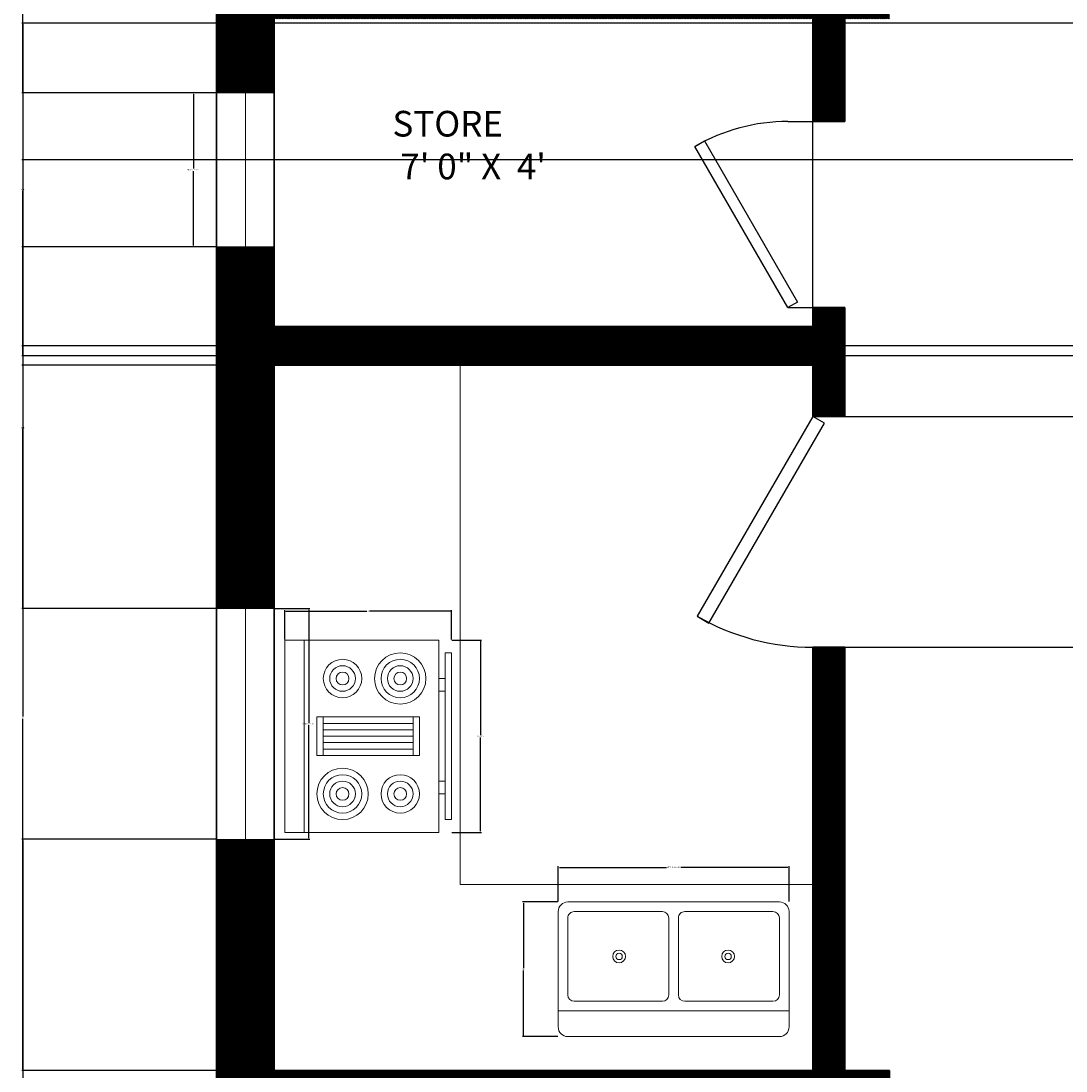
# Model space of a CAD drawing. Units: inches. Extents: x -24 to 516, y -23 to 640.
# Tile 2 of 5: x -24 to 139, y 288 to 452. Entities that reach past the tile are written whole.
import ezdxf

# ---------------------------------------------------------------- set-up
doc = ezdxf.new("R2010")
doc.units = ezdxf.units.IN
doc.header["$MEASUREMENT"] = 0
for name, color, linetype, lineweight in [('A-ANNO-DIMS', 2, 'Continuous', 18), ('A-AREA-IDEN', 7, 'Continuous', 18), ('A-WALL', 7, 'Continuous', 35), ('doors', 40, 'Continuous', 25), ('kitchen', 181, 'Continuous', 18), ('window', 30, 'Continuous', 18)]:
    doc.layers.add(name, color=color, linetype=linetype, lineweight=lineweight)
doc.layers.add('A-WALL-PATT', color=198, linetype='Continuous', lineweight=13, true_color=0x2e0f2e)
doc.styles.get("Standard").update_dxf_attribs({"font": 'arial.ttf'})
doc.dimstyles.get("Standard").update_dxf_attribs({"dimtxt": 0.18, "dimasz": 0.18, "dimexe": 0.18, "dimexo": 0.0625, "dimgap": 0.09, "dimtad": 0, "dimtih": 1, "dimtoh": 1, "dimdec": 4, "dimzin": 0, "dimdsep": 46, "dimtxsty": 'Standard', "dimcen": 0.09, "dimadec": 0, "dimazin": 0, "dimtfac": 1, "dimtdec": 4, "dimtofl": 0, "dimtmove": 0, "dimatfit": 3, "dimfxl": 1, "dimtolj": 1, "dimtzin": 0, "dimarcsym": 0})

# ---------------------------------------------------------------- blocks, each defined once
blk = doc.blocks.new('*U6')
for p, q in [((0, 0), (0, -100)), ((750, 0), (750, -100))]:
    blk.add_line(p, q)
blk.add_lwpolyline([(0, 0), (649.5, 375), (671.4, 337.1), (21.9, -37.9)], close=True)
blk.add_arc((0, 0), 750, 0, 30)
blk = doc.blocks.new('*U7')
for p, q in [((0, 0), (0, 100)), ((750, 0), (750, 100))]:
    blk.add_line(p, q)
blk.add_lwpolyline([(0, 0), (649.5, -375), (671.4, -337.1), (21.9, 37.9)], close=True)
blk.add_arc((0, 0), 750, 330, 0)
blk = doc.blocks.new('Range-Oven - 30 in top')
for p, q in [((0, -3), (30, -3)), ((12, -6), (18, -6)), ((13, -20), (13, -6)), ((14, -6), (14, -20)), ((15, -20), (15, -6)), ((16, -6), (16, -20)), ((17, -20), (17, -6)), ((18, -20), (12, -20)), ((6, -24), (6, -25)), ((8, -25), (8, -24)), ((22, -25), (22, -24)), ((24, -24), (24, -25))]:
    blk.add_line(p, q)
for points in [[(0, -24), (0, 0), (30, 0), (30, -24)], [(12, -21), (12, -5), (18, -5), (18, -21)], [(2, -26), (2, -25), (28, -25), (28, -26)]]:
    blk.add_lwpolyline(points, close=True)
for centre, radius in [((6, -9), 4), ((6, -9), 3), ((24, -9), 3), ((6, -9), 2), ((6, -9), 1), ((24, -9), 2), ((24, -9), 1), ((24, -18), 4), ((6, -18), 3), ((6, -18), 2), ((24, -18), 3), ((24, -18), 2), ((6, -18), 1), ((24, -18), 1)]:
    blk.add_circle(centre, radius)
blk = doc.blocks.new('Sink-double - 36 in top')
for p, q in [((-18, -4), (18, -4)), ((-0.75, -18.5), (-0.75, -6.5)), ((0.75, -6.5), (0.75, -18.5))]:
    blk.add_line(p, q)
for points in [[(-16.5, 0), (16.5, 0)], [(-18, -19.5), (-18, -1.5)], [(18, -1.5), (18, -19.5)], [(-16.5, -18.5), (-16.5, -6.5)], [(-15.5, -5.5), (-1.75, -5.5)], [(1.75, -5.5), (15.5, -5.5)], [(16.5, -6.5), (16.5, -18.5)], [(-1.75, -19.5), (-15.5, -19.5)], [(15.5, -19.5), (1.75, -19.5)], [(16.5, -21), (-16.5, -21)]]:
    blk.add_lwpolyline(points)
for centre, radius in [((-8.5, -12.5), 1), ((-8.5, -12.5), 0.5), ((8.5, -12.5), 1), ((8.5, -12.5), 0.5)]:
    blk.add_circle(centre, radius)
for centre, radius, start, end in [((-16.5, -1.5), 1.5, 90, 180), ((16.5, -1.5), 1.5, 0, 90), ((-15.5, -6.5), 1, 90, 180), ((-1.75, -6.5), 1, 0, 90), ((1.75, -6.5), 1, 90, 180), ((15.5, -6.5), 1, 0, 90), ((-16.5, -19.5), 1.5, 180, 270), ((-15.5, -18.5), 1, 180, 270), ((-1.75, -18.5), 1, 270, 0), ((1.75, -18.5), 1, 180, 270), ((15.5, -18.5), 1, 270, 0), ((16.5, -19.5), 1.5, 270, 0)]:
    blk.add_arc(centre, radius, start, end)
blk = doc.blocks.new('WIN-36IN')
for p, q in [((0, 0), (0, 36)), ((0, 36), (9, 36)), ((4.5, 0), (4.5, 36)), ((9, 36), (9, 0)), ((9, 0), (0, 0)), ((9, 0), (4.5, 0))]:
    blk.add_line(p, q)
blk = doc.blocks.new('WIN-24IN')
for p, q in [((0, 0), (0, 24)), ((0, 24), (9, 24)), ((4.5, 0), (4.5, 24)), ((9, 24), (9, 0)), ((9, 0), (0, 0)), ((9, 0), (4.5, 0))]:
    blk.add_line(p, q)
blk = doc.blocks.new('*D19')
at = {"layer": 'A-ANNO-DIMS', "color": 0, "lineweight": -2, "transparency": 16777216}
for p, q in [((15.15, 360.05), (20.67, 360.05)), ((20.49, 359.87), (20.49, 342.23)), ((20.49, 324.23), (20.49, 341.86)), ((15.15, 324.05), (20.67, 324.05))]:
    blk.add_line(p, q, dxfattribs=at)
at = {"layer": 'A-ANNO-DIMS', "color": 0, "transparency": 16777216}
for points in [[(20.46, 359.87), (20.52, 359.87), (20.49, 360.05)], [(20.46, 324.23), (20.52, 324.23), (20.49, 324.05)]]:
    blk.add_solid(points, dxfattribs=at)
at = {"layer": 'Defpoints', "color": 0, "transparency": 16777216}
for p in [(15.09, 360.05), (20.49, 360.05), (15.09, 324.05)]:
    blk.add_point(p, dxfattribs=at)
at = {"layer": 'A-ANNO-DIMS', "color": 0, "transparency": 16777216, "insert": (20.49, 342.05), "char_height": 0.18, "attachment_point": 5}
blk.add_mtext('\\A1;WINDOW 36 TYP.', dxfattribs=at)
blk = doc.blocks.new('*D20')
at = {"layer": 'A-ANNO-DIMS', "color": 0, "lineweight": -2, "transparency": 16777216}
for p, q in [((6.09, 323.98), (6.09, 318.47)), ((15.09, 323.98), (15.09, 318.47)), ((6.27, 318.65), (10.13, 318.65)), ((14.91, 318.65), (11.05, 318.65))]:
    blk.add_line(p, q, dxfattribs=at)
at = {"layer": 'A-ANNO-DIMS', "color": 0, "transparency": 16777216}
for points in [[(6.27, 318.68), (6.27, 318.62), (6.09, 318.65)], [(14.91, 318.68), (14.91, 318.62), (15.09, 318.65)]]:
    blk.add_solid(points, dxfattribs=at)
at = {"layer": 'Defpoints', "color": 0, "transparency": 16777216}
for p in [(6.09, 324.05), (15.09, 324.05), (15.09, 318.65)]:
    blk.add_point(p, dxfattribs=at)
at = {"layer": 'A-ANNO-DIMS', "color": 0, "transparency": 16777216, "insert": (10.59, 318.65), "char_height": 0.18, "attachment_point": 5}
blk.add_mtext('\\A1;9 TYP.', dxfattribs=at)
blk = doc.blocks.new('*D21')
at = {"layer": 'A-ANNO-DIMS', "color": 0, "lineweight": -2, "transparency": 16777216}
for p, q in [((6.03, 440.47), (2.31, 440.47)), ((2.49, 440.29), (2.49, 428.66)), ((2.49, 416.65), (2.49, 428.29)), ((6.03, 416.47), (2.31, 416.47))]:
    blk.add_line(p, q, dxfattribs=at)
at = {"layer": 'A-ANNO-DIMS', "color": 0, "transparency": 16777216}
for points in [[(2.46, 440.29), (2.52, 440.29), (2.49, 440.47)], [(2.46, 416.65), (2.52, 416.65), (2.49, 416.47)]]:
    blk.add_solid(points, dxfattribs=at)
at = {"layer": 'Defpoints', "color": 0, "transparency": 16777216}
for p in [(2.49, 440.47), (6.09, 440.47), (6.09, 416.47)]:
    blk.add_point(p, dxfattribs=at)
at = {"layer": 'A-ANNO-DIMS', "color": 0, "transparency": 16777216, "insert": (2.49, 428.47), "char_height": 0.18, "attachment_point": 5}
blk.add_mtext('\\A1;WINDOW 24 TYP.', dxfattribs=at)
blk = doc.blocks.new('*D22')
at = {"layer": 'A-ANNO-DIMS', "color": 0, "lineweight": -2, "transparency": 16777216}
for p, q in [((6.09, 440.54), (6.09, 444.25)), ((6.27, 444.07), (10.13, 444.07)), ((14.91, 444.07), (11.05, 444.07)), ((15.09, 440.54), (15.09, 444.25))]:
    blk.add_line(p, q, dxfattribs=at)
at = {"layer": 'A-ANNO-DIMS', "color": 0, "transparency": 16777216}
for points in [[(6.27, 444.1), (6.27, 444.04), (6.09, 444.07)], [(14.91, 444.1), (14.91, 444.04), (15.09, 444.07)]]:
    blk.add_solid(points, dxfattribs=at)
at = {"layer": 'Defpoints', "color": 0, "transparency": 16777216}
for p in [(15.09, 444.07), (6.09, 440.47), (15.09, 440.47)]:
    blk.add_point(p, dxfattribs=at)
at = {"layer": 'A-ANNO-DIMS', "color": 0, "transparency": 16777216, "insert": (10.59, 444.07), "char_height": 0.18, "attachment_point": 5}
blk.add_mtext('\\A1;9 TYP.', dxfattribs=at)
blk = doc.blocks.new('*D27')
at = {"layer": 'A-ANNO-DIMS', "color": 0, "lineweight": -2, "transparency": 16777216}
for p, q in [((42.81, 355.13), (47.43, 355.13)), ((47.25, 354.95), (47.25, 340.32)), ((47.25, 325.31), (47.25, 339.95)), ((42.81, 325.13), (47.43, 325.13))]:
    blk.add_line(p, q, dxfattribs=at)
at = {"layer": 'A-ANNO-DIMS', "color": 0, "transparency": 16777216}
for points in [[(47.22, 354.95), (47.28, 354.95), (47.25, 355.13)], [(47.22, 325.31), (47.28, 325.31), (47.25, 325.13)]]:
    blk.add_solid(points, dxfattribs=at)
at = {"layer": 'Defpoints', "color": 0, "transparency": 16777216}
for p in [(42.75, 355.13), (47.25, 355.13), (42.75, 325.13)]:
    blk.add_point(p, dxfattribs=at)
at = {"layer": 'A-ANNO-DIMS', "color": 0, "transparency": 16777216, "insert": (47.25, 340.13), "char_height": 0.18, "attachment_point": 5}
blk.add_mtext('\\A1;RANGE 30', dxfattribs=at)
blk = doc.blocks.new('*D28')
at = {"layer": 'A-ANNO-DIMS', "color": 0, "lineweight": -2, "transparency": 16777216}
for p, q in [((16.75, 355.2), (16.75, 359.81)), ((16.93, 359.63), (29.53, 359.63)), ((42.57, 359.63), (29.97, 359.63)), ((42.75, 355.2), (42.75, 359.81))]:
    blk.add_line(p, q, dxfattribs=at)
at = {"layer": 'A-ANNO-DIMS', "color": 0, "transparency": 16777216}
for points in [[(16.93, 359.66), (16.93, 359.6), (16.75, 359.63)], [(42.57, 359.66), (42.57, 359.6), (42.75, 359.63)]]:
    blk.add_solid(points, dxfattribs=at)
at = {"layer": 'Defpoints', "color": 0, "transparency": 16777216}
for p in [(16.75, 359.63), (16.75, 355.13), (42.75, 355.13)]:
    blk.add_point(p, dxfattribs=at)
at = {"layer": 'A-ANNO-DIMS', "color": 0, "transparency": 16777216, "insert": (29.75, 359.63), "char_height": 0.18, "attachment_point": 5}
blk.add_mtext('\\A1;26', dxfattribs=at)
blk = doc.blocks.new('*D29')
at = {"layer": 'A-ANNO-DIMS', "color": 0, "lineweight": -2, "transparency": 16777216}
for p, q in [((59.39, 314.35), (59.39, 319.86)), ((59.57, 319.68), (76.26, 319.68)), ((95.21, 319.68), (78.52, 319.68)), ((95.39, 314.35), (95.39, 319.86))]:
    blk.add_line(p, q, dxfattribs=at)
at = {"layer": 'A-ANNO-DIMS', "color": 0, "transparency": 16777216}
for points in [[(59.57, 319.71), (59.57, 319.65), (59.39, 319.68)], [(95.21, 319.71), (95.21, 319.65), (95.39, 319.68)]]:
    blk.add_solid(points, dxfattribs=at)
at = {"layer": 'Defpoints', "color": 0, "transparency": 16777216}
for p in [(59.39, 319.68), (59.39, 314.28), (95.39, 314.28)]:
    blk.add_point(p, dxfattribs=at)
at = {"layer": 'A-ANNO-DIMS', "color": 0, "transparency": 16777216, "insert": (77.39, 319.68), "char_height": 0.18, "attachment_point": 5}
blk.add_mtext('\\A1;KITCHEN SINK 36', dxfattribs=at)
blk = doc.blocks.new('*D30')
at = {"layer": 'A-ANNO-DIMS', "color": 0, "lineweight": -2, "transparency": 16777216}
for p, q in [((59.33, 314.28), (53.81, 314.28)), ((53.99, 314.1), (53.99, 303.96)), ((53.99, 293.46), (53.99, 303.6)), ((59.33, 293.28), (53.81, 293.28))]:
    blk.add_line(p, q, dxfattribs=at)
at = {"layer": 'A-ANNO-DIMS', "color": 0, "transparency": 16777216}
for points in [[(53.96, 314.1), (54.02, 314.1), (53.99, 314.28)], [(53.96, 293.46), (54.02, 293.46), (53.99, 293.28)]]:
    blk.add_solid(points, dxfattribs=at)
at = {"layer": 'Defpoints', "color": 0, "transparency": 16777216}
for p in [(59.39, 314.28), (53.99, 293.28), (59.39, 293.28)]:
    blk.add_point(p, dxfattribs=at)
at = {"layer": 'A-ANNO-DIMS', "color": 0, "transparency": 16777216, "insert": (53.99, 303.78), "char_height": 0.18, "attachment_point": 5}
blk.add_mtext('\\A1;21', dxfattribs=at)
blk = doc.blocks.new('*D42')
at = {"layer": 'A-ANNO-DIMS', "color": 0, "lineweight": -2, "transparency": 16777216}
for p, q in [((6.03, 324.05), (-24.28, 324.05)), ((-24.1, 323.87), (-24.1, 278.18)), ((-24.1, 232.13), (-24.1, 277.81)), ((6.03, 231.95), (-24.28, 231.95))]:
    blk.add_line(p, q, dxfattribs=at)
at = {"layer": 'A-ANNO-DIMS', "color": 0, "transparency": 16777216}
for points in [[(-24.13, 323.87), (-24.07, 323.87), (-24.1, 324.05)], [(-24.13, 232.13), (-24.07, 232.13), (-24.1, 231.95)]]:
    blk.add_solid(points, dxfattribs=at)
at = {"layer": 'Defpoints', "color": 0, "transparency": 16777216}
for p in [(-24.1, 324.05), (6.09, 324.05), (6.09, 231.95)]:
    blk.add_point(p, dxfattribs=at)
at = {"layer": 'A-ANNO-DIMS', "color": 0, "transparency": 16777216, "insert": (-24.1, 278), "char_height": 0.18, "attachment_point": 5}
blk.add_mtext('\\A1;92.1', dxfattribs=at)
blk = doc.blocks.new('*D43')
at = {"layer": 'A-ANNO-DIMS', "color": 0, "lineweight": -2, "transparency": 16777216}
for p, q in [((6.03, 416.47), (-24.28, 416.47)), ((-24.1, 416.29), (-24.1, 388.44)), ((-24.1, 360.23), (-24.1, 388.08)), ((6.03, 360.05), (-24.28, 360.05))]:
    blk.add_line(p, q, dxfattribs=at)
at = {"layer": 'A-ANNO-DIMS', "color": 0, "transparency": 16777216}
for points in [[(-24.13, 416.29), (-24.07, 416.29), (-24.1, 416.47)], [(-24.13, 360.23), (-24.07, 360.23), (-24.1, 360.05)]]:
    blk.add_solid(points, dxfattribs=at)
at = {"layer": 'Defpoints', "color": 0, "transparency": 16777216}
for p in [(-24.1, 416.47), (6.09, 416.47), (6.09, 360.05)]:
    blk.add_point(p, dxfattribs=at)
at = {"layer": 'A-ANNO-DIMS', "color": 0, "transparency": 16777216, "insert": (-24.1, 388.26), "char_height": 0.18, "attachment_point": 5}
blk.add_mtext('\\A1;56.43', dxfattribs=at)
blk = doc.blocks.new('*D44')
at = {"layer": 'A-ANNO-DIMS', "color": 0, "lineweight": -2, "transparency": 16777216}
for p, q in [((6.03, 518.75), (-24.28, 518.75)), ((-24.1, 518.57), (-24.1, 479.8)), ((-24.1, 440.65), (-24.1, 479.43)), ((6.03, 440.47), (-24.28, 440.47))]:
    blk.add_line(p, q, dxfattribs=at)
at = {"layer": 'A-ANNO-DIMS', "color": 0, "transparency": 16777216}
for points in [[(-24.13, 518.57), (-24.07, 518.57), (-24.1, 518.75)], [(-24.13, 440.65), (-24.07, 440.65), (-24.1, 440.47)]]:
    blk.add_solid(points, dxfattribs=at)
at = {"layer": 'Defpoints', "color": 0, "transparency": 16777216}
for p in [(-24.1, 518.75), (6.09, 518.75), (6.09, 440.47)]:
    blk.add_point(p, dxfattribs=at)
at = {"layer": 'A-ANNO-DIMS', "color": 0, "transparency": 16777216, "insert": (-24.1, 479.61), "char_height": 0.18, "attachment_point": 5}
blk.add_mtext('\\A1;78.28', dxfattribs=at)
blk = doc.blocks.new('*D46')
at = {"layer": 'A-ANNO-DIMS', "color": 0, "lineweight": -2, "transparency": 16777216}
for p, q in [((15.09, 398.08), (15.09, 640.38)), ((99.09, 398.08), (99.09, 640.38)), ((15.27, 640.2), (56.87, 640.2)), ((98.91, 640.2), (57.31, 640.2))]:
    blk.add_line(p, q, dxfattribs=at)
at = {"layer": 'A-ANNO-DIMS', "color": 0, "transparency": 16777216}
for points in [[(15.27, 640.23), (15.27, 640.17), (15.09, 640.2)], [(98.91, 640.23), (98.91, 640.17), (99.09, 640.2)]]:
    blk.add_solid(points, dxfattribs=at)
at = {"layer": 'Defpoints', "color": 0, "transparency": 16777216}
for p in [(99.09, 640.2), (15.09, 398.01), (99.09, 398.01)]:
    blk.add_point(p, dxfattribs=at)
at = {"layer": 'A-ANNO-DIMS', "color": 0, "transparency": 16777216, "insert": (57.09, 640.2), "char_height": 0.18, "attachment_point": 5}
blk.add_mtext('\\A1;84', dxfattribs=at)
blk = doc.blocks.new('*D47')
at = {"layer": 'A-ANNO-DIMS', "color": 0, "lineweight": -2, "transparency": 16777216}
for p, q in [((15.03, 398.01), (-24.28, 398.01)), ((-24.1, 397.83), (-24.1, 343.2)), ((-24.1, 288.19), (-24.1, 342.83)), ((15.03, 288.01), (-24.28, 288.01))]:
    blk.add_line(p, q, dxfattribs=at)
at = {"layer": 'A-ANNO-DIMS', "color": 0, "transparency": 16777216}
for points in [[(-24.13, 397.83), (-24.07, 397.83), (-24.1, 398.01)], [(-24.13, 288.19), (-24.07, 288.19), (-24.1, 288.01)]]:
    blk.add_solid(points, dxfattribs=at)
at = {"layer": 'Defpoints', "color": 0, "transparency": 16777216}
for p in [(-24.1, 398.01), (15.09, 398.01), (15.09, 288.01)]:
    blk.add_point(p, dxfattribs=at)
at = {"layer": 'A-ANNO-DIMS', "color": 0, "transparency": 16777216, "insert": (-24.1, 343.01), "char_height": 0.18, "attachment_point": 5}
blk.add_mtext('\\A1;110', dxfattribs=at)
blk = doc.blocks.new('*D48')
at = {"layer": 'A-ANNO-DIMS', "color": 0, "lineweight": -2, "transparency": 16777216}
for p, q in [((99.15, 390.01), (516.45, 390.01)), ((516.27, 389.83), (516.27, 372.2)), ((516.27, 354.19), (516.27, 371.83)), ((99.15, 354.01), (516.45, 354.01))]:
    blk.add_line(p, q, dxfattribs=at)
at = {"layer": 'A-ANNO-DIMS', "color": 0, "transparency": 16777216}
for points in [[(516.24, 389.83), (516.3, 389.83), (516.27, 390.01)], [(516.24, 354.19), (516.3, 354.19), (516.27, 354.01)]]:
    blk.add_solid(points, dxfattribs=at)
at = {"layer": 'Defpoints', "color": 0, "transparency": 16777216}
for p in [(99.09, 390.01), (516.27, 390.01), (99.09, 354.01)]:
    blk.add_point(p, dxfattribs=at)
at = {"layer": 'A-ANNO-DIMS', "color": 0, "transparency": 16777216, "insert": (516.27, 372.01), "char_height": 0.18, "attachment_point": 5}
blk.add_mtext('\\A1;36', dxfattribs=at)
blk = doc.blocks.new('*D52')
at = {"layer": 'A-ANNO-DIMS', "color": 0, "lineweight": -2, "transparency": 16777216}
for p, q in [((392.03, 430.01), (-24.28, 430.01)), ((-24.1, 429.83), (-24.1, 415.7)), ((-24.1, 401.19), (-24.1, 415.33)), ((392.03, 401.01), (-24.28, 401.01))]:
    blk.add_line(p, q, dxfattribs=at)
at = {"layer": 'A-ANNO-DIMS', "color": 0, "transparency": 16777216}
for points in [[(-24.13, 429.83), (-24.07, 429.83), (-24.1, 430.01)], [(-24.13, 401.19), (-24.07, 401.19), (-24.1, 401.01)]]:
    blk.add_solid(points, dxfattribs=at)
at = {"layer": 'Defpoints', "color": 0, "transparency": 16777216}
for p in [(-24.1, 430.01), (392.09, 430.01), (392.09, 401.01)]:
    blk.add_point(p, dxfattribs=at)
at = {"layer": 'A-ANNO-DIMS', "color": 0, "transparency": 16777216, "insert": (-24.1, 415.51), "char_height": 0.18, "attachment_point": 5}
blk.add_mtext('\\A1;29', dxfattribs=at)
blk = doc.blocks.new('*D56')
at = {"layer": 'A-ANNO-DIMS', "color": 0, "lineweight": -2, "transparency": 16777216}
for p, q in [((218.16, 451.37), (-24.28, 451.37)), ((-24.1, 451.19), (-24.1, 425.59)), ((-24.1, 399.62), (-24.1, 425.22)), ((197.45, 399.44), (-24.28, 399.44))]:
    blk.add_line(p, q, dxfattribs=at)
at = {"layer": 'A-ANNO-DIMS', "color": 0, "transparency": 16777216}
for points in [[(-24.13, 451.19), (-24.07, 451.19), (-24.1, 451.37)], [(-24.13, 399.62), (-24.07, 399.62), (-24.1, 399.44)]]:
    blk.add_solid(points, dxfattribs=at)
at = {"layer": 'Defpoints', "color": 0, "transparency": 16777216}
for p in [(218.23, 451.37), (-24.1, 399.44), (197.51, 399.44)]:
    blk.add_point(p, dxfattribs=at)
at = {"layer": 'A-ANNO-DIMS', "color": 0, "transparency": 16777216, "insert": (-24.1, 425.4), "char_height": 0.18, "attachment_point": 5}
blk.add_mtext('\\A1;51.92', dxfattribs=at)

msp = doc.modelspace()

# ---------------------------------------------------------------- hatches: boundary and pattern name
at = {"layer": 'A-WALL-PATT'}
h = msp.add_hatch(dxfattribs=at)
h.set_pattern_fill('ANSI31', color=256)
h.set_pattern_definition([(45, (-12045.43418, -42625.98622), (-0.08838834765, 0.08838834765), [])])
h.paths.add_polyline_path([(161.63, 139.013), (155.088, 139.013), (155.088, 283.013), (203.088, 283.013), (203.088, 171.013), (208.088, 171.013), (208.088, 283.013), (211.088, 283.013), (211.088, 288.013), (208.088, 288.013), (147.088, 288.013), (147.088, 283.013), (150.088, 283.013), (150.088, 139.013), (87.664, 139.013), (87.664, 134.513), (87.664, 130.013), (161.63, 130.013)])
h.paths.add_polyline_path([(256.352, 139.013), (208.088, 139.013), (208.088, 142.013), (203.088, 142.013), (203.088, 139.013), (185.63, 139.013), (185.63, 130.013), (256.352, 130.013)])
h.paths.add_polyline_path([(345.088, 326.013), (336.088, 326.013), (336.088, 288.013), (247.088, 288.013), (247.088, 283.013), (340.088, 283.013), (340.088, 139.013), (292.352, 139.013), (292.352, 134.513), (292.352, 130.013), (345.088, 130.013)])
h.paths.add_polyline_path([(51.664, 139.013), (15.088, 139.013), (15.088, 195.946), (10.588, 195.946), (6.088, 195.946), (6.088, 130.013), (51.664, 130.013)])
h.paths.add_polyline_path([(15.088, 283.013), (111.088, 283.013), (111.088, 288.013), (104.088, 288.013), (104.088, 354.013), (99.088, 354.013), (99.088, 288.013), (15.088, 288.013), (15.088, 324.046), (10.588, 324.046), (6.088, 324.046), (6.088, 231.946), (15.088, 231.946)])
h.paths.add_polyline_path([(15.088, 398.013), (99.088, 398.013), (99.088, 390.013), (104.088, 390.013), (104.088, 393.013), (104.088, 407.013), (99.088, 407.013), (99.088, 404.013), (15.088, 404.013), (15.088, 416.474), (10.588, 416.474), (6.088, 416.474), (6.088, 360.046), (15.088, 360.046)])
h.paths.add_polyline_path([(15.088, 518.753), (10.588, 518.753), (6.088, 518.753), (6.088, 440.474), (15.088, 440.474), (15.088, 452.013), (99.088, 452.013), (99.088, 436.013), (104.088, 436.013), (104.088, 452.013), (111.088, 452.013), (111.088, 457.013), (15.088, 457.013)])

# ---------------------------------------------------------------- linework, layer by layer
at = {"layer": 'A-WALL'}
for p, q in [((15.088, 404.013), (15.088, 452.013)), ((99.088, 436.013), (99.088, 452.013)), ((104.088, 436.013), (104.088, 452.013)), ((104.088, 436.013), (99.088, 436.013)), ((99.088, 404.013), (99.088, 407.013)), ((99.088, 404.013), (99.088, 407.013)), ((99.088, 407.013), (104.088, 407.013)), ((104.088, 390.013), (104.088, 407.013)), ((15.088, 404.013), (99.088, 404.013)), ((15.088, 398.013), (99.088, 398.013)), ((15.088, 288.013), (15.088, 398.013)), ((99.088, 390.013), (99.088, 398.013)), ((104.088, 393.013), (104.088, 390.013)), ((104.088, 390.013), (99.088, 390.013)), ((99.088, 288.013), (99.088, 354.013)), ((104.088, 354.013), (99.088, 354.013)), ((104.088, 288.013), (104.088, 354.013)), ((15.088, 288.013), (99.088, 288.013)), ((99.088, 288.013), (15.088, 288.013)), ((104.088, 288.013), (111.088, 288.013)), ((111.088, 288.013), (104.088, 288.013)), ((111.088, 283.013), (111.088, 288.013))]:
    msp.add_line(p, q, dxfattribs=at)
msp.add_lwpolyline([(345.088, 130.013), (6.088, 130.013), (6.088, 610.013), (486.088, 610.013), (486.088, 173.013)], dxfattribs=at)
at = {"layer": 'kitchen'}
msp.add_line((99.088, 288.013), (99.088, 317.013), dxfattribs=at)
msp.add_lwpolyline([(99.088, 317.013), (44.088, 317.013), (44.088, 398.013)], dxfattribs=at)

# ---------------------------------------------------------------- block references
at = {"layer": 'doors'}
for name, p, xscale, yscale, zscale, rotation in [('*U6', (95.222, 407.013), 0.0386666666666677, 0.0386666666666677, 0.0386666666666677, 90), ('*U7', (99.088, 390.013), 0.0480000000000013, 0.0480000000000013, 0.0480000000000013, 270)]:
    msp.add_blockref(name, p, dxfattribs=dict(at, xscale=xscale, yscale=yscale, zscale=zscale, rotation=rotation))
at = {"layer": 'kitchen'}
for name, p, rotation in [('Range-Oven - 30 in top', (16.75, 325.133), 89.99999999999999), ('Sink-double - 36 in top', (77.389, 293.283), 180)]:
    msp.add_blockref(name, p, dxfattribs=dict(at, rotation=rotation))
at = {"layer": 'window'}
for name, p in [('WIN-24IN', (6.088, 416.474)), ('WIN-36IN', (6.088, 324.046))]:
    msp.add_blockref(name, p, dxfattribs=at)

# ---------------------------------------------------------------- texts
at = {"layer": 'A-AREA-IDEN', "insert": (31.092, 437.666), "char_height": 4, "attachment_point": 1}
msp.add_mtext_dynamic_manual_height_columns('  STORE\\P   7\' 0" X  4\'', width=74.82673, gutter_width=1, heights=[0], dxfattribs=at)

# ---------------------------------------------------------------- dimensions: what is measured, and where the dimension line sits
at = {"layer": 'A-ANNO-DIMS'}
dim = msp.add_linear_dim(base=(99.088, 640.198), p1=(15.088, 398.013), p2=(99.088, 398.013), dimstyle='Standard', override={"dimdec": 0, "dimlfac": 1, "dimrnd": 0, "dimzin": 0, "dimdsep": 46, "dimlunit": 2}, dxfattribs=at)
dim.commit()
dim.dimension.update_dxf_attribs({"geometry": '*D46', "text_midpoint": (57.088, 640.198)})
for base, p1, p2, angle, override, picture, middle in [((-24.097, 518.753), (6.088, 440.474), (6.088, 518.753), 90, {"dimdec": 2, "dimlfac": 1, "dimrnd": 0, "dimzin": 0, "dimdsep": 46, "dimlunit": 2}, '*D44', (-24.097, 479.614)), ((-24.097, 399.442), (218.226, 451.366), (197.509, 399.442), 90, {"dimdec": 2, "dimlfac": 1, "dimrnd": 0, "dimzin": 0, "dimdsep": 46, "dimlunit": 2}, '*D56', (-24.097, 425.404)), ((-24.097, 430.013), (392.088, 401.013), (392.088, 430.013), 90, {"dimdec": 0, "dimlfac": 1, "dimrnd": 0, "dimzin": 0, "dimdsep": 46, "dimlunit": 2}, '*D52', (-24.097, 415.513)), ((-24.097, 416.474), (6.088, 360.046), (6.088, 416.474), 90, {"dimdec": 2, "dimlfac": 1, "dimrnd": 0, "dimzin": 0, "dimdsep": 46, "dimlunit": 2}, '*D43', (-24.097, 388.26)), ((-24.097, 398.013), (15.088, 288.013), (15.088, 398.013), 90, {"dimdec": 0, "dimlfac": 1, "dimrnd": 0, "dimzin": 0, "dimdsep": 46, "dimlunit": 2}, '*D47', (-24.097, 343.013)), ((516.273, 390.013), (99.088, 354.013), (99.088, 390.013), 90, {"dimdec": 0, "dimlfac": 1, "dimrnd": 0, "dimzin": 0, "dimdsep": 46, "dimlunit": 2}, '*D48', (516.273, 372.013)), ((16.75, 359.633), (42.75, 355.133), (16.75, 355.133), 180, {"dimdec": 0, "dimlfac": 1, "dimrnd": 0, "dimzin": 0, "dimdsep": 46, "dimlunit": 2}, '*D28', (29.75, 359.633)), ((-24.097, 324.046), (6.088, 231.946), (6.088, 324.046), 90, {"dimdec": 1, "dimlfac": 1, "dimrnd": 0, "dimzin": 0, "dimdsep": 46, "dimlunit": 2}, '*D42', (-24.097, 277.996)), ((53.989, 293.283), (59.389, 314.283), (59.389, 293.283), 270, {"dimdec": 0, "dimlfac": 1, "dimrnd": 0, "dimzin": 0, "dimdsep": 46, "dimlunit": 2}, '*D30', (53.989, 303.783))]:
    dim = msp.add_linear_dim(base=base, p1=p1, p2=p2, angle=angle, dimstyle='Standard', override=override, dxfattribs=at)
    dim.commit()
    dim.dimension.update_dxf_attribs({"geometry": picture, "text_midpoint": middle})
for base, p1, p2, picture, middle in [((15.088, 444.074), (6.088, 440.474), (15.088, 440.474), '*D22', (10.588, 444.074)), ((15.088, 318.646), (6.088, 324.046), (15.088, 324.046), '*D20', (10.588, 318.646))]:
    dim = msp.add_linear_dim(base=base, p1=p1, p2=p2, text='<> TYP.', dimstyle='Standard', override={"dimdec": 0, "dimlfac": 1, "dimrnd": 0, "dimzin": 0, "dimdsep": 46, "dimlunit": 2}, dxfattribs=at)
    dim.commit()
    dim.dimension.update_dxf_attribs({"geometry": picture, "text_midpoint": middle})
for base, p1, p2, angle, text, picture, middle in [((2.488, 440.474), (6.088, 416.474), (6.088, 440.474), 90, 'WINDOW <> TYP.', '*D21', (2.488, 428.474)), ((20.488, 360.046), (15.088, 324.046), (15.088, 360.046), 90, 'WINDOW <> TYP.', '*D19', (20.488, 342.046)), ((47.25, 355.133), (42.75, 325.133), (42.75, 355.133), 90, 'RANGE <>', '*D27', (47.25, 340.133)), ((59.389, 319.683), (95.389, 314.283), (59.389, 314.283), 180, 'KITCHEN SINK <>', '*D29', (77.389, 319.683))]:
    dim = msp.add_linear_dim(base=base, p1=p1, p2=p2, angle=angle, text=text, dimstyle='Standard', override={"dimdec": 0, "dimlfac": 1, "dimrnd": 0, "dimzin": 0, "dimdsep": 46, "dimlunit": 2}, dxfattribs=at)
    dim.commit()
    dim.dimension.update_dxf_attribs({"geometry": picture, "text_midpoint": middle})

doc.saveas('drawing.dxf')
